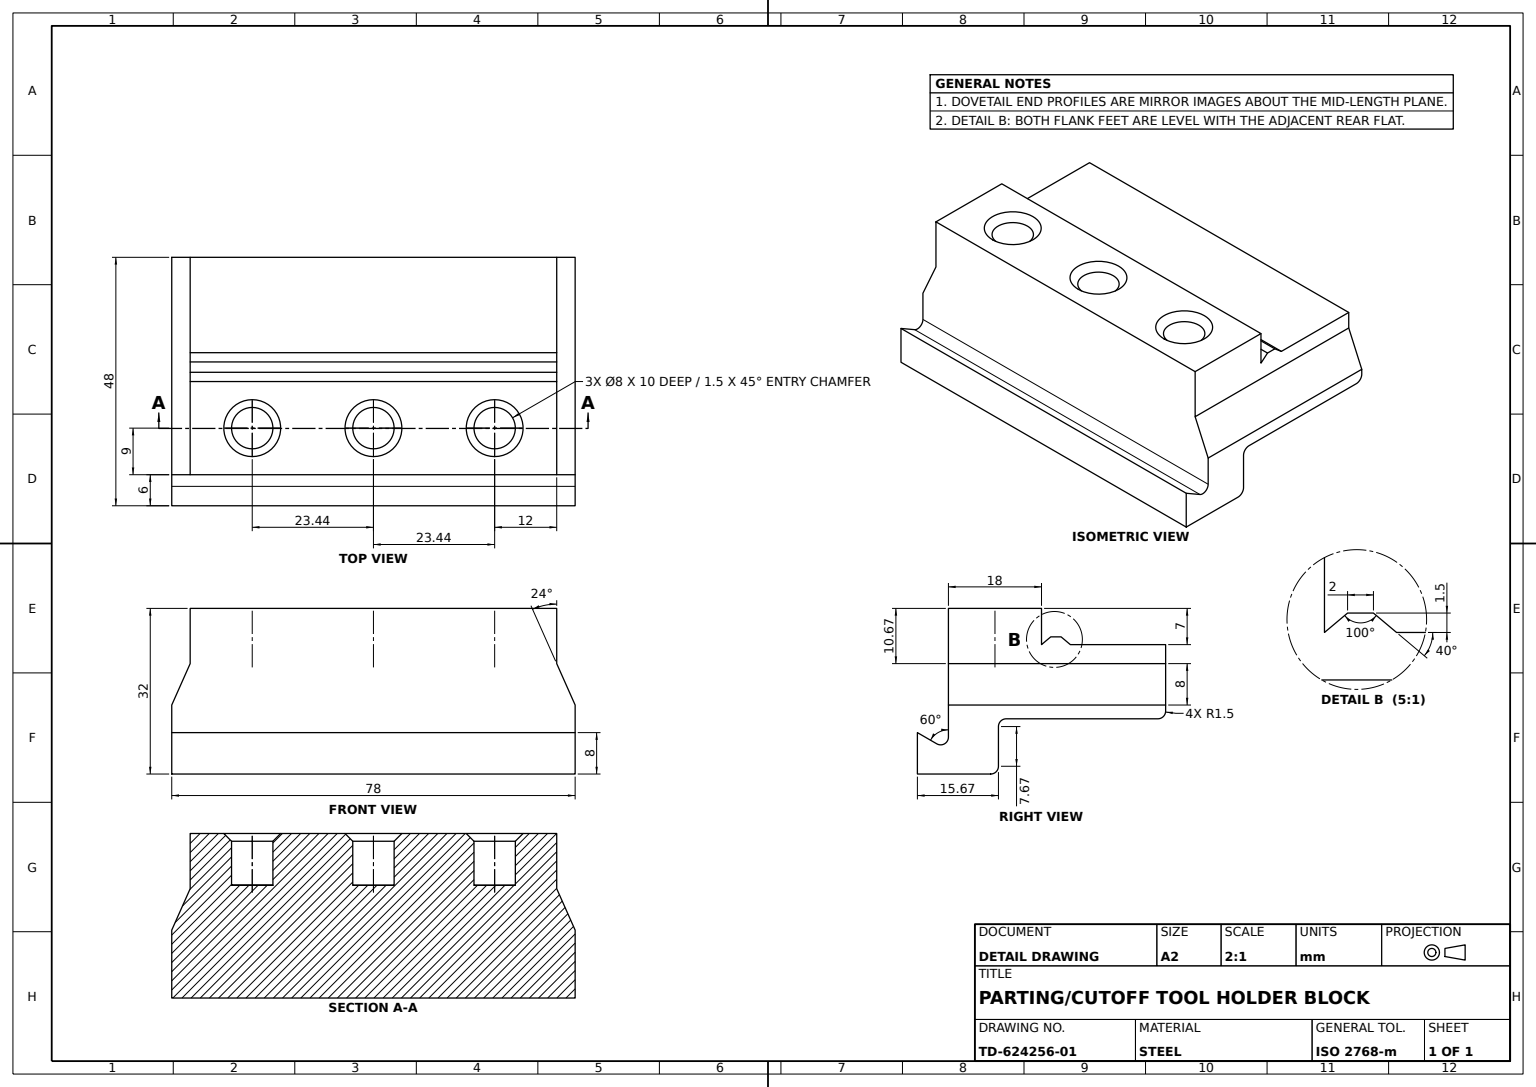
SolidWorks part; units mm, degrees
material "Plain Carbon Steel"
ref_plane "Front Plane" through (0, 0, 0) normal (0, 0, 1) x (1, 0, 0)
ref_plane "Top Plane" through (0, 0, 0) normal (0, 1, 0) x (1, 0, 0)
ref_plane "Right Plane" through (0, 0, 0) normal (1, 0, 0) x (0, 0, -1)
sketch "Dovetail Body Profile" plane through (0, 0, 0) normal (0, 0, 1) x (1, 0, 0)
  line L0 (0, 0) -> (0, 13.33)
  line L1 (0, 13.33) -> (3.5618, 21.33)
  line L2 (3.5618, 21.33) -> (3.5618, 32)
  line L3 (3.5618, 32) -> (74.4382, 32)
  line L4 (74.4382, 32) -> (74.4382, 21.33)
  line L5 (74.4382, 21.33) -> (78, 13.33)
  line L6 (78, 13.33) -> (78, 0)
  line L7 (78, 0) -> (0, 0)
  dimension "D1" = 32
  dimension "D2" = 78
  dimension "D3" = 24
  dimension "D4" = 24
  dimension "D5" = 8
  dimension "D6" = 8
  dimension "D7" = 10.67
  dimension "D8" = 10.67
extrude "Dovetail Body" add sketch "Dovetail Body Profile" against normal blind 48
sketch "Groove Profile" plane through (78, 0, 0) normal (1, 0, 0) x (0, 0, -1)
  line L1 (0, 0) -> (0, 13.33) construction
  line L2 (0, 8) -> (3.75, 5.8349)
  line L3 (6, 7.134) -> (6, 32)
  line L4 (48, 32) -> (0, 32) construction
  line L6 (48, 25) -> (48, 32)
  line L7 (48, 32) -> (24, 32)
  line L8 (0, 32) -> (0, 8)
  line L9 (0, 1.5) -> (0, 0)
  line L10 (24, 32) -> (24, 25)
  line L11 (24, 25) -> (25.7876, 26.5)
  line L12 (25.7876, 26.5) -> (27.7876, 26.5)
  line L13 (27.7876, 26.5) -> (29.5753, 25)
  line L14 (29.5753, 25) -> (48, 25)
  line L15 (48, 12.17) -> (48, 10.67)
  line L16 (46.5, 10.67) -> (17.1714, 10.67)
  line L17 (15.6714, 9.17) -> (15.6714, 1.5)
  line L18 (6, 32) -> (0, 32)
  line L19 (0, 0) -> (1.5, 0)
  line L20 (14.1714, 0) -> (48, 0)
  line L21 (48, 0) -> (48, 12.17)
  arc A0 (3.75, 5.8349) -> (6, 7.134) centre (4.5, 7.134) ccw
  arc A1 (1.5, 0) -> (0, 1.5) centre (1.5, 1.5) cw
  arc A2 (48, 12.17) -> (46.5, 10.67) centre (46.5, 12.17) cw
  arc A3 (15.6714, 9.17) -> (17.1714, 10.67) centre (17.1714, 9.17) cw
  arc A4 (14.1714, 0) -> (15.6714, 1.5) centre (14.1714, 1.5) ccw
  point P19 (0, 0)
  dimension "D4" = 1.5
  dimension "D12" = 1.5
  dimension "D1" = 60
  dimension "D2" = 18
  dimension "D3" = 8
  dimension "D5" = 100
  dimension "D6" = 40
  dimension "D7" = 2
  dimension "D8" = 1.5
  dimension "D9" = 1.5
  dimension "D10" = 7
  dimension "D11" = 6
  dimension "D13" = 10.67
  dimension "D14" = 1.5
  dimension "D15" = 7.67
  dimension "D16" = 15.6714
extrude "Groove Cut" cut sketch "Groove Profile" against normal blind 88 contours L8 L2 A0 L3 L18 | L7 L10 L11 L12 L13 L14 L6 | A2 L16 A3 L17 A4 L20 L21
sketch "Mounting Holes Layout" plane through (0, 32, 0) normal (0, 1, 0) x (1, 0, 0)
  line L0 (3.5618, 15) -> (74.4382, 15) construction
  line L1 (3.5618, 24) -> (3.5618, 6) construction
  line L2 (74.4382, 24) -> (74.4382, 6) construction
  line L3 (39, 24) -> (39, 6) construction
  line L4 (3.5618, 24) -> (74.4382, 24) construction
  line L5 (0, 6) -> (78, 6) construction
  circle A0 centre (62.4382, 15) radius 4
  circle A1 centre (39, 15) radius 4
  circle A2 centre (15.5618, 15) radius 4
  dimension "D3" = 8
  dimension "D4" = 8
  dimension "D5" = 8
  dimension "D1" = 12
  dimension "D2" = 12
extrude "Mounting Holes 3xØ8" cut sketch "Mounting Holes Layout" against normal blind 10
chamfer "Hole Chamfers 1.5x45" distance 1.5 angle 45 3 edges at (62.4382, 32, -11) (39, 32, -11) (15.5618, 32, -11)
